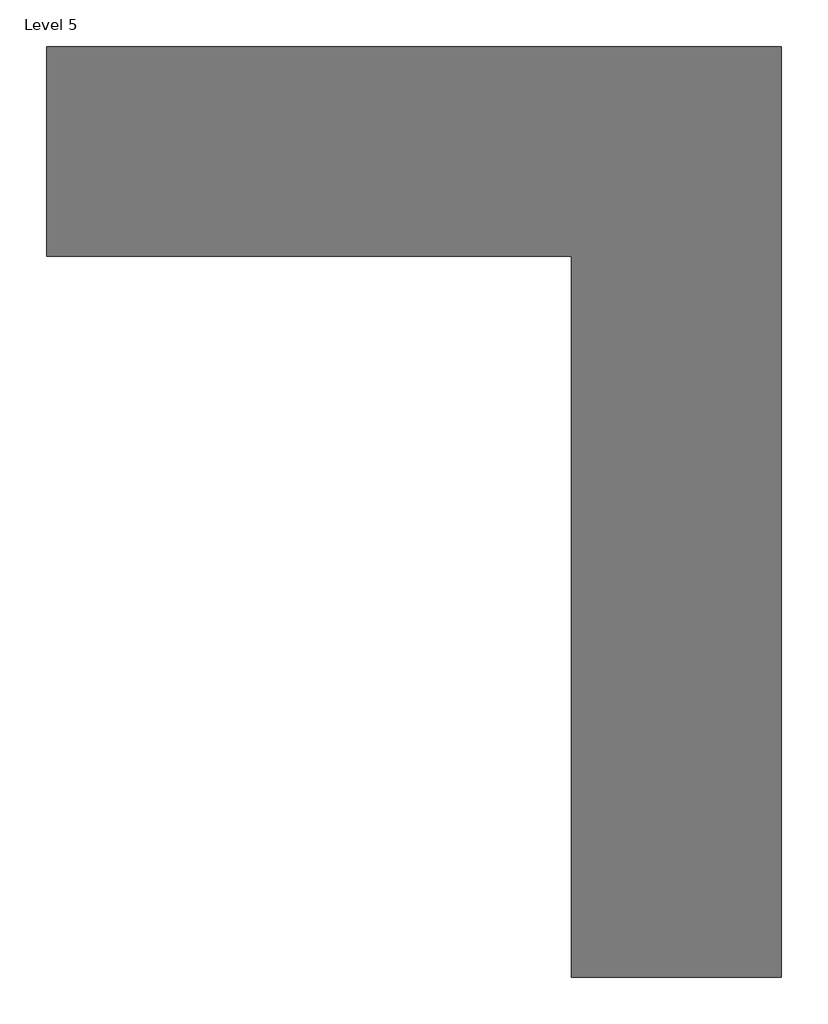
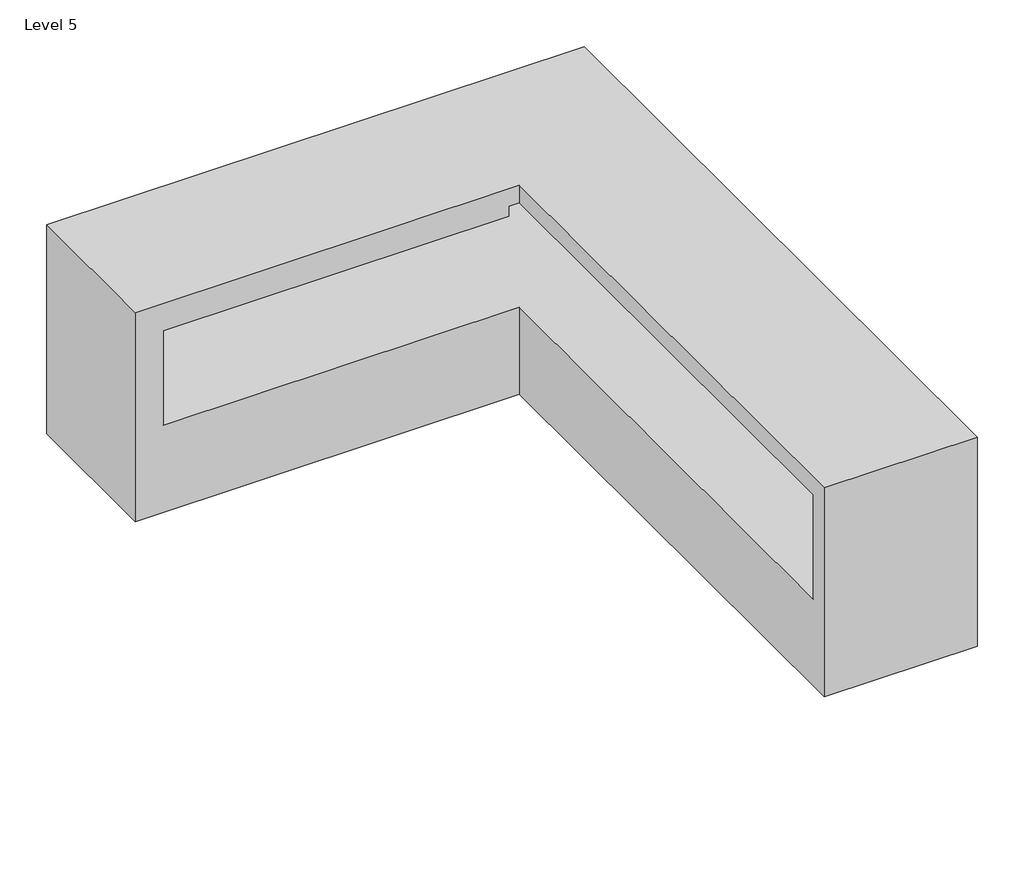
# One storey: 1 proxy.
"""IFC4 building model written with IfcOpenShell, lengths in millimetres."""

from ifc_helpers import new_model, si_unit, origin, place, context, project, spatial, transform, mapped, element, save
from components import kitchen_1_kitchen_1_5a132608

model = new_model("IFC4")

# Units and contexts
model_context = context("Model", 3, world=origin())
ifc_project = project(units=[si_unit("LENGTHUNIT", "METRE", prefix="MILLI")], contexts=[model_context])

# Site, building, storey
site = spatial("IfcSite", under=ifc_project)
building = spatial("IfcBuilding", under=site)
storey = spatial("IfcBuildingStorey", under=building, Name="Level 5", Elevation=-609.6)

# Proxy
placement = place(None, origin())
kitchen_1_kitchen_1_shape = kitchen_1_kitchen_1_5a132608(model_context)
element("IfcBuildingElementProxy", 1, Name="kitchen 1 : kitchen 1", ObjectType="kitchen 1 : kitchen 1", at=placement, inside=storey, context=model_context, shape_type="MappedRepresentation", body=[
    mapped(kitchen_1_kitchen_1_shape, transform((0.0, 0.0, 0.0), x_axis=(1.0, 0.0, 0.0), y_axis=(0.0, 1.0, 0.0), z_axis=(0.0, 0.0, 1.0))),
])

save(model, "model.ifc")

# Revit data of these elements
# Element 1 (IfcBuildingElementProxy, "kitchen 1 : kitchen 1")
#   Phase Created = New Construction
